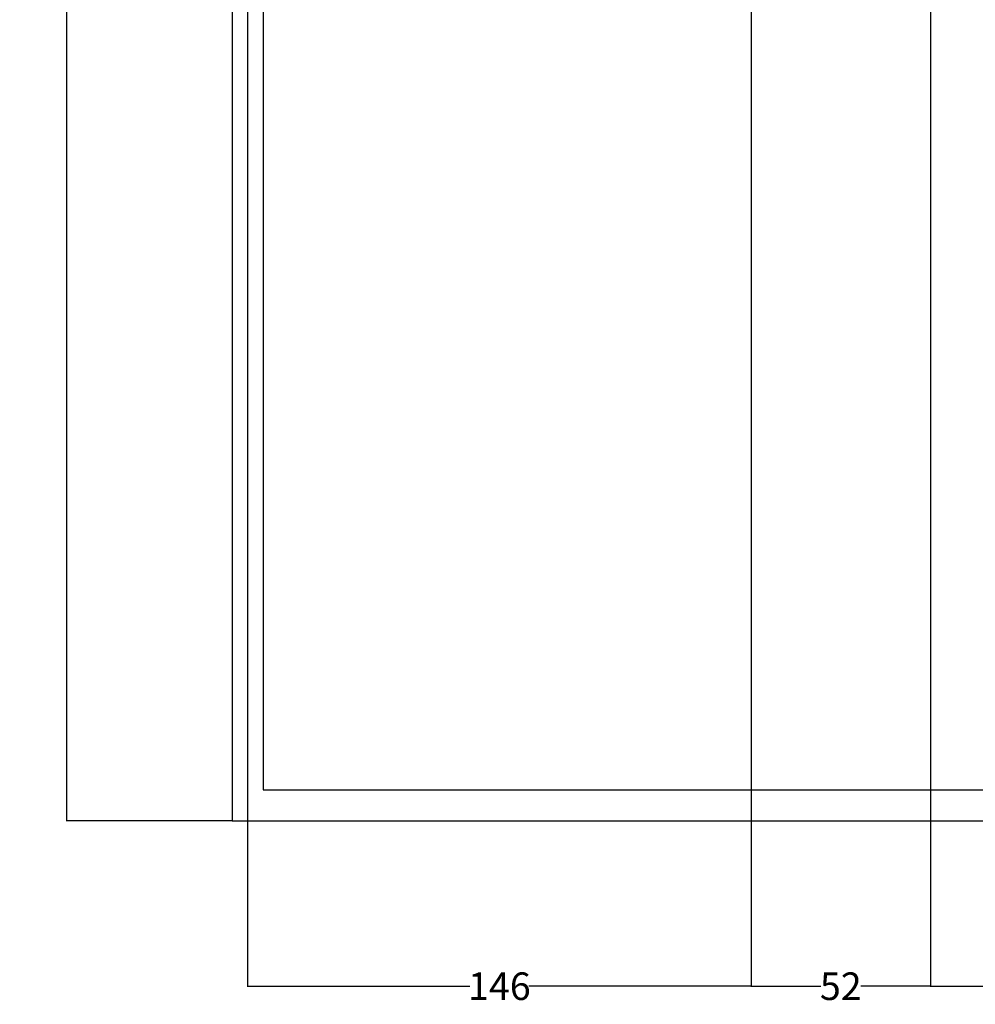
# Model space of a CAD drawing. Units: inches. Extents: x -48 to 50072, y 0 to 21068.
# Tile 57 of 75: x 697 to 974, y 232 to 517. Entities that reach past the tile are written whole.
import ezdxf

# ---------------------------------------------------------------- set-up
doc = ezdxf.new("R2010")
doc.units = ezdxf.units.IN
doc.header["$MEASUREMENT"] = 0
doc.linetypes.add('ACAD_ISO02W100', pattern=[15, 12, -3])
for name, color, linetype, lineweight in [('A-ANNO-DIMS', 2, 'Continuous', 18), ('C-PROP', 7, 'Continuous', 25), ('C-PROP-REF', 32, 'ACAD_ISO02W100', 13)]:
    doc.layers.add(name, color=color, linetype=linetype, lineweight=lineweight)
doc.styles.get("Standard").update_dxf_attribs({"font": 'arial.ttf'})
doc.dimstyles.get("Standard").update_dxf_attribs({"dimtxt": 8, "dimasz": 0.18, "dimexe": 0.18, "dimexo": 0.0625, "dimgap": 0.09, "dimtad": 0, "dimtih": 1, "dimtoh": 1, "dimdec": 1, "dimzin": 0, "dimdsep": 46, "dimlunit": 4, "dimtxsty": 'Standard', "dimblk": 'ARCHTICK', "dimcen": 0.09, "dimadec": 0, "dimazin": 0, "dimtfac": 1, "dimtdec": 1, "dimtofl": 0, "dimtmove": 0, "dimatfit": 3, "dimldrblk": 'ARCHTICK', "dimfxl": 1, "dimtolj": 1, "dimtzin": 0, "dimarcsym": 0})

# ---------------------------------------------------------------- blocks, each defined once
blk = doc.blocks.new('_ArchTick')
at = {"color": 0, "linetype": 'ByBlock', "const_width": 0.15}
blk.add_lwpolyline([(-0.5, -0.5), (0.5, 0.5)], dxfattribs=at)
blk = doc.blocks.new('*D130')
at = {"layer": 'A-ANNO-DIMS', "color": 0, "lineweight": -2, "transparency": 16777216}
for p, q in [((758.7, 1241.46), (710.63, 1241.46)), ((710.81, 1241.46), (710.81, 767.29)), ((710.81, 284.76), (710.81, 758.94)), ((758.7, 284.76), (710.63, 284.76))]:
    blk.add_line(p, q, dxfattribs=at)
at = {"layer": 'Defpoints', "color": 0, "transparency": 16777216}
for p in [(710.81, 1241.46), (758.76, 1241.46), (758.76, 284.76)]:
    blk.add_point(p, dxfattribs=at)
at = {"layer": 'A-ANNO-DIMS', "color": 0, "lineweight": -2, "transparency": 16777216, "xscale": 0.18, "yscale": 0.18, "zscale": 0.18}
for p, rotation in [((710.81, 1241.46), 90), ((710.81, 284.76), 270)]:
    blk.add_blockref('_ArchTick', p, dxfattribs=dict(at, rotation=rotation))
at = {"layer": 'A-ANNO-DIMS', "color": 0, "transparency": 16777216, "insert": (710.81, 763.11), "char_height": 8, "attachment_point": 5}
blk.add_mtext('\\A1;956.7', dxfattribs=at)
blk = doc.blocks.new('*D135')
at = {"layer": 'A-ANNO-DIMS', "color": 0, "lineweight": -2, "transparency": 16777216}
for p, q in [((763.26, 748.4), (763.26, 236.63)), ((909.26, 748.4), (909.26, 236.63)), ((763.26, 236.81), (827.71, 236.81)), ((909.26, 236.81), (844.81, 236.81))]:
    blk.add_line(p, q, dxfattribs=at)
at = {"layer": 'Defpoints', "color": 0, "transparency": 16777216}
for p in [(763.26, 748.46), (909.26, 748.46), (909.26, 236.81)]:
    blk.add_point(p, dxfattribs=at)
at = {"layer": 'A-ANNO-DIMS', "color": 0, "lineweight": -2, "transparency": 16777216, "xscale": 0.18, "yscale": 0.18, "zscale": 0.18, "rotation": 180}
blk.add_blockref('_ArchTick', (763.26, 236.81), dxfattribs=at)
at = {"layer": 'A-ANNO-DIMS', "color": 0, "lineweight": -2, "transparency": 16777216, "xscale": 0.18, "yscale": 0.18, "zscale": 0.18}
blk.add_blockref('_ArchTick', (909.26, 236.81), dxfattribs=at)
at = {"layer": 'A-ANNO-DIMS', "color": 0, "transparency": 16777216, "insert": (836.26, 236.81), "char_height": 8, "attachment_point": 5}
blk.add_mtext('\\A1;146', dxfattribs=at)
blk = doc.blocks.new('*D136')
at = {"layer": 'A-ANNO-DIMS', "color": 0, "lineweight": -2, "transparency": 16777216}
for p, q in [((909.26, 748.4), (909.26, 236.63)), ((961.26, 559.4), (961.26, 236.63)), ((909.26, 236.81), (929.48, 236.81)), ((961.26, 236.81), (941.04, 236.81))]:
    blk.add_line(p, q, dxfattribs=at)
at = {"layer": 'Defpoints', "color": 0, "transparency": 16777216}
for p in [(909.26, 748.46), (961.26, 559.46), (961.26, 236.81)]:
    blk.add_point(p, dxfattribs=at)
at = {"layer": 'A-ANNO-DIMS', "color": 0, "lineweight": -2, "transparency": 16777216, "xscale": 0.18, "yscale": 0.18, "zscale": 0.18, "rotation": 180}
blk.add_blockref('_ArchTick', (909.26, 236.81), dxfattribs=at)
at = {"layer": 'A-ANNO-DIMS', "color": 0, "lineweight": -2, "transparency": 16777216, "xscale": 0.18, "yscale": 0.18, "zscale": 0.18}
blk.add_blockref('_ArchTick', (961.26, 236.81), dxfattribs=at)
at = {"layer": 'A-ANNO-DIMS', "color": 0, "transparency": 16777216, "insert": (935.26, 236.81), "char_height": 8, "attachment_point": 5}
blk.add_mtext('\\A1;52', dxfattribs=at)
blk = doc.blocks.new('*D137')
at = {"layer": 'A-ANNO-DIMS', "color": 0, "lineweight": -2, "transparency": 16777216}
for p, q in [((961.26, 559.4), (961.26, 236.63)), ((1042.26, 559.4), (1042.26, 236.63)), ((961.26, 236.81), (996.71, 236.81)), ((1042.26, 236.81), (1006.81, 236.81))]:
    blk.add_line(p, q, dxfattribs=at)
at = {"layer": 'Defpoints', "color": 0, "transparency": 16777216}
for p in [(961.26, 559.46), (1042.26, 559.46), (1042.26, 236.81)]:
    blk.add_point(p, dxfattribs=at)
at = {"layer": 'A-ANNO-DIMS', "color": 0, "lineweight": -2, "transparency": 16777216, "xscale": 0.18, "yscale": 0.18, "zscale": 0.18, "rotation": 180}
blk.add_blockref('_ArchTick', (961.26, 236.81), dxfattribs=at)
at = {"layer": 'A-ANNO-DIMS', "color": 0, "lineweight": -2, "transparency": 16777216, "xscale": 0.18, "yscale": 0.18, "zscale": 0.18}
blk.add_blockref('_ArchTick', (1042.26, 236.81), dxfattribs=at)
at = {"layer": 'A-ANNO-DIMS', "color": 0, "transparency": 16777216, "insert": (1001.76, 236.81), "char_height": 8, "attachment_point": 5}
blk.add_mtext('\\A1;81', dxfattribs=at)

msp = doc.modelspace()

# ---------------------------------------------------------------- linework, layer by layer
at = {"layer": 'C-PROP'}
for p, q in [((758.761, 1241.464), (758.761, 284.764)), ((767.761, 931.464), (767.761, 293.764)), ((767.761, 293.764), (1289.761, 293.764)), ((758.761, 284.764), (1298.761, 284.764))]:
    msp.add_line(p, q, dxfattribs=at)
at = {"layer": 'C-PROP-REF'}
msp.add_line((763.261, 1236.964), (763.261, 284.764), dxfattribs=at)

# ---------------------------------------------------------------- dimensions: what is measured, and where the dimension line sits
at = {"layer": 'A-ANNO-DIMS'}
dim = msp.add_linear_dim(base=(710.811, 1241.464), p1=(758.761, 284.764), p2=(758.761, 1241.464), angle=90, dimstyle='Standard', override={"dimdec": 1, "dimlfac": 1, "dimrnd": 0, "dimzin": 0, "dimdsep": 46, "dimlunit": 2}, dxfattribs=at)
dim.commit()
dim.dimension.update_dxf_attribs({"geometry": '*D130', "text_midpoint": (710.811, 763.114)})
for base, p1, p2, picture, middle in [((909.261, 236.814), (763.261, 748.464), (909.261, 748.464), '*D135', (836.261, 236.814)), ((961.261, 236.814), (909.261, 748.464), (961.261, 559.464), '*D136', (935.261, 236.814)), ((1042.261, 236.814), (961.261, 559.464), (1042.261, 559.464), '*D137', (1001.761, 236.814))]:
    dim = msp.add_linear_dim(base=base, p1=p1, p2=p2, dimstyle='Standard', override={"dimdec": 0, "dimlfac": 1, "dimrnd": 0, "dimzin": 0, "dimdsep": 46, "dimlunit": 2}, dxfattribs=at)
    dim.commit()
    dim.dimension.update_dxf_attribs({"geometry": picture, "text_midpoint": middle})

doc.saveas('drawing.dxf')
